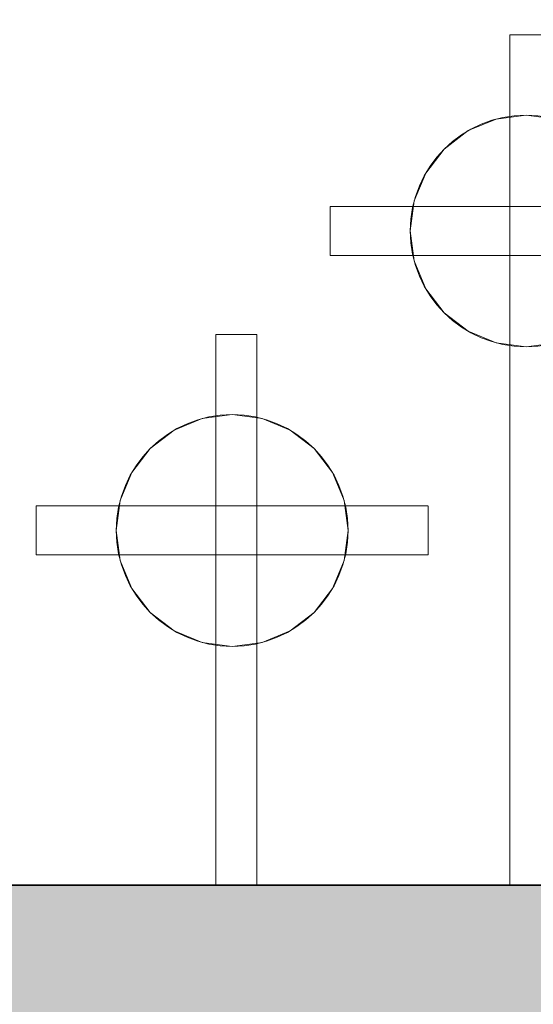
# Model space of a CAD drawing. Units: inches. Extents: x 2696 to 3240, y 1564 to 2310.
# Tile 30 of 76: x 3142.316 to 3146.244, y 1698.791 to 1706.319. Entities that reach past the tile are written whole.
import ezdxf

# ---------------------------------------------------------------- set-up
doc = ezdxf.new("R2010")
doc.units = ezdxf.units.IN
for name, color, linetype, lineweight in [('A-ANNO-DIMS', 3, 'Continuous', 18), ('A-FLOR-FIXT', 8, 'Continuous', 18), ('A-FURN', 251, 'Continuous', 13), ('A-WALL', 7, 'Continuous', 35), ('A-WALL-PATT', 9, 'Continuous', 13)]:
    doc.layers.add(name, color=color, linetype=linetype, lineweight=lineweight)
doc.layers.add('FURNITURE', color=250, linetype='Continuous')
doc.styles.add('TIMES NEW', font='times.ttf')
doc.dimstyles.new('Siddhuu', dxfattribs={"dimtxt": 6, "dimasz": 2.5, "dimexe": 1.25, "dimexo": 0.625, "dimtad": 1, "dimdec": 1, "dimlunit": 4, "dimtxsty": 'TIMES NEW', "dimcen": 2.5, "dimclrd": 256, "dimclre": 1, "dimclrt": 7, "dimadec": 0, "dimazin": 0, "dimtfac": 1, "dimtdec": 1, "dimtmove": 0, "dimatfit": 3, "dimfxl": 1, "dimtolj": 1, "dimlwd": -1, "dimarcsym": 0})

# ---------------------------------------------------------------- blocks, each defined once
blk = doc.blocks.new('A$C1af1f523')
at = {"layer": 'A-FURN'}
for p, q in [((-2.9003, 3.9351), (-2.9003, 0.9365)), ((-2.9003, 3.9351, 0.5), (-2.9003, 0.9365, 0.5)), ((-2.9003, 3.9351), (-2.9003, 3.9351, 0.5)), ((-2.5253, 3.9351), (-2.9003, 3.9351)), ((-2.5253, 3.9351, 0.5), (-2.9003, 3.9351, 0.5)), ((-2.5253, 3.9351), (-2.5253, 0.9365)), ((-2.5253, 3.9351, 0.5), (-2.5253, 0.9365, 0.5)), ((-2.5253, 3.9351), (-2.5253, 3.9351, 0.5)), ((-2.7128, 3.3215), (-2.7128, 3.3215, 0.5)), ((-2.9421, 3.2913), (-2.9421, 3.2913, 0.5)), ((-2.4835, 3.2913), (-2.4835, 3.2913, 0.5)), ((-3.1558, 3.2028), (-3.1558, 3.2028, 0.5)), ((-2.2698, 3.2028), (-2.2698, 3.2028, 0.5)), ((-3.3393, 3.062), (-3.3393, 3.062, 0.5)), ((-2.0863, 3.062), (-2.0863, 3.062, 0.5)), ((-3.4801, 2.8785), (-3.4801, 2.8785, 0.5)), ((-1.9455, 2.8785), (-1.9455, 2.8785, 0.5)), ((-3.5686, 2.6648), (-3.5686, 2.6648, 0.5)), ((-1.857, 2.6648), (-1.857, 2.6648, 0.5)), ((0, 2.5605), (-4.2116, 2.5605)), ((0, 2.5605, 0.5), (-4.2116, 2.5605, 0.5)), ((-4.2116, 2.5605), (-4.2116, 2.5605, 0.5)), ((-4.2116, 2.5594), (-4.2116, 2.248)), ((-4.2116, 2.5594, 0.5), (-4.2116, 2.248, 0.5)), ((-4.2116, 2.5594), (-4.2116, 2.5594, 0.5)), ((-3.5988, 2.4355), (-3.5988, 2.4355, 0.5)), ((-1.8268, 2.4355), (-1.8268, 2.4355, 0.5)), ((0, 2.248), (-4.2116, 2.248)), ((0, 2.248, 0.5), (-4.2116, 2.248, 0.5)), ((-4.2116, 2.248), (-4.2116, 2.248, 0.5)), ((-4.2116, 2.248), (-4.2116, 2.2469)), ((-4.2116, 2.248, 0.5), (-4.2116, 2.2469, 0.5)), ((-4.2116, 2.2469), (-4.2116, 2.2469, 0.5)), ((-3.5686, 2.2061), (-3.5686, 2.2061, 0.5)), ((-1.857, 2.2061), (-1.857, 2.2061, 0.5)), ((-3.4801, 1.9924), (-3.4801, 1.9924, 0.5)), ((-1.9455, 1.9924), (-1.9455, 1.9924, 0.5)), ((-3.3393, 1.8089), (-3.3393, 1.8089, 0.5)), ((-2.0863, 1.8089), (-2.0863, 1.8089, 0.5)), ((-4.8156, 1.6871), (-5.1906, 1.6871)), ((-4.8156, 1.6871, 0.5), (-5.1906, 1.6871, 0.5)), ((-5.1906, 1.6871), (-5.1906, 1.6871, 0.5)), ((-5.1906, 1.6871), (-5.1901, -1.3115)), ((-5.1906, 1.6871, 0.5), (-5.1901, -1.3115, 0.5)), ((-4.8156, 1.6871), (-4.8156, 1.6871, 0.5)), ((-4.8156, 1.6871), (-4.8151, -1.3115)), ((-4.8156, 1.6871, 0.5), (-4.8151, -1.3115, 0.5)), ((-3.1558, 1.6681), (-3.1558, 1.6681, 0.5)), ((-2.2698, 1.6681), (-2.2698, 1.6681, 0.5)), ((-2.9421, 1.5796), (-2.9421, 1.5796, 0.5)), ((-2.7128, 1.5494), (-2.7128, 1.5494, 0.5)), ((-2.4835, 1.5796), (-2.4835, 1.5796, 0.5)), ((-5.0026, 1.0735), (-5.0026, 1.0735, 0.5)), ((-5.232, 1.0433), (-5.232, 1.0433, 0.5)), ((-4.7733, 1.0433), (-4.7733, 1.0433, 0.5)), ((-5.4457, 0.9548), (-5.4457, 0.9548, 0.5)), ((-4.5596, 0.9548), (-4.5596, 0.9548, 0.5)), ((-2.9003, 0.9365), (-2.9003, 0.9365, 0.5)), ((-2.5253, 0.9365), (-2.8979, 0.9365)), ((-2.5253, 0.9365, 0.5), (-2.8979, 0.9365, 0.5)), ((-2.8979, 0.9365), (-2.8979, 0.9365, 0.5)), ((-2.5253, 0.9365), (-2.5253, 0.9365, 0.5)), ((-5.6292, 0.814), (-5.6292, 0.814, 0.5)), ((-4.3761, 0.814), (-4.3761, 0.814, 0.5)), ((-5.77, 0.6305), (-5.77, 0.6305, 0.5)), ((-4.2353, 0.6305), (-4.2353, 0.6305, 0.5)), ((-5.8585, 0.4168), (-5.8585, 0.4168, 0.5)), ((-4.1468, 0.4168), (-4.1468, 0.4168, 0.5)), ((0, 0.3125), (-6.5015, 0.3125)), ((0, 0.3125, 0.5), (-6.5015, 0.3125, 0.5)), ((-6.5015, 0.3125), (-6.5015, 0.3125, 0.5)), ((-6.5015, 0.3114), (-6.5015, 0)), ((-6.5015, 0.3114, 0.5), (-6.5015, 0, 0.5)), ((-6.5015, 0.3114), (-6.5015, 0.3114, 0.5)), ((-5.8887, 0.1875), (-5.8887, 0.1875, 0.5)), ((-4.1166, 0.1875), (-4.1166, 0.1875, 0.5))]:
    blk.add_line(p, q, dxfattribs=at)
for centre in [(-2.7128, 2.4355), (-2.7128, 2.4355, 0.5), (-5.0026, 0.1875), (-5.0026, 0.1875, 0.5)]:
    blk.add_circle(centre, 0.886, dxfattribs=at)
at = {"layer": 'FURNITURE'}
for p, q in [((0, 2.5605), (0, 2.5605, 0.5)), ((0, 2.248), (0, 2.248, 0.5)), ((0, 0.3125), (0, 0.3125, 0.5))]:
    blk.add_line(p, q, dxfattribs=at)
at = {"layer": 'A-FURN'}
mesh = blk.add_polyface(dxfattribs=at)
corners = [(-2.9003, 0.9365, 0.5), (-2.9003, 3.9351), (-2.9003, 0.9365), (-2.9003, 3.9351, 0.5)]
mesh.append_faces([[corners[k] for k in face] for face in [(2, 1, 0), (3, 0, 1)]], dxfattribs={"vtx1": -1})
mesh = blk.add_polyface(dxfattribs=at)
corners = [(-2.5253, 3.9351, 0.5), (-2.9003, 3.9351), (-2.9003, 3.9351, 0.5), (-2.5253, 3.9351)]
mesh.append_faces([[corners[k] for k in face] for face in [(2, 1, 0), (3, 0, 1)]], dxfattribs={"vtx1": -1})
mesh = blk.add_polyface(dxfattribs=at)
corners = [(-2.5253, 0.9365, 0.5), (-2.5253, 3.9351), (-2.5253, 0.9365), (-2.5253, 3.9351, 0.5)]
mesh.append_faces([[corners[k] for k in face] for face in [(2, 1, 0), (3, 0, 1)]], dxfattribs={"vtx1": -1})
mesh = blk.add_polyface(dxfattribs=at)
corners = [(-2.7128, 3.3215), (-2.9421, 3.2913, 0.5), (-2.9421, 3.2913), (-2.7128, 3.3215, 0.5)]
mesh.append_faces([[corners[k] for k in face] for face in [(2, 1, 0), (3, 0, 1)]], dxfattribs={"vtx1": -1})
mesh = blk.add_polyface(dxfattribs=at)
corners = [(-2.4835, 3.2913), (-2.7128, 3.3215, 0.5), (-2.7128, 3.3215), (-2.4835, 3.2913, 0.5)]
mesh.append_faces([[corners[k] for k in face] for face in [(2, 1, 0), (3, 0, 1)]], dxfattribs={"vtx1": -1})
mesh = blk.add_polyface(dxfattribs=at)
corners = [(-2.9421, 3.2913), (-3.1558, 3.2028, 0.5), (-3.1558, 3.2028), (-2.9421, 3.2913, 0.5)]
mesh.append_faces([[corners[k] for k in face] for face in [(2, 1, 0), (3, 0, 1)]], dxfattribs={"vtx1": -1})
mesh = blk.add_polyface(dxfattribs=at)
corners = [(-2.2698, 3.2028), (-2.4835, 3.2913, 0.5), (-2.4835, 3.2913), (-2.2698, 3.2028, 0.5)]
mesh.append_faces([[corners[k] for k in face] for face in [(2, 1, 0), (3, 0, 1)]], dxfattribs={"vtx1": -1})
mesh = blk.add_polyface(dxfattribs=at)
corners = [(-3.1558, 3.2028), (-3.3393, 3.062, 0.5), (-3.3393, 3.062), (-3.1558, 3.2028, 0.5)]
mesh.append_faces([[corners[k] for k in face] for face in [(2, 1, 0), (3, 0, 1)]], dxfattribs={"vtx1": -1})
mesh = blk.add_polyface(dxfattribs=at)
corners = [(-2.0863, 3.062), (-2.2698, 3.2028, 0.5), (-2.2698, 3.2028), (-2.0863, 3.062, 0.5)]
mesh.append_faces([[corners[k] for k in face] for face in [(2, 1, 0), (3, 0, 1)]], dxfattribs={"vtx1": -1})
mesh = blk.add_polyface(dxfattribs=at)
corners = [(-3.3393, 3.062, 0.5), (-3.4801, 2.8785), (-3.3393, 3.062), (-3.4801, 2.8785, 0.5)]
mesh.append_faces([[corners[k] for k in face] for face in [(2, 1, 0), (3, 0, 1)]], dxfattribs={"vtx1": -1})
mesh = blk.add_polyface(dxfattribs=at)
corners = [(-1.9455, 2.8785, 0.5), (-2.0863, 3.062), (-1.9455, 2.8785), (-2.0863, 3.062, 0.5)]
mesh.append_faces([[corners[k] for k in face] for face in [(2, 1, 0), (3, 0, 1)]], dxfattribs={"vtx1": -1})
mesh = blk.add_polyface(dxfattribs=at)
corners = [(-3.4801, 2.8785, 0.5), (-3.5686, 2.6648), (-3.4801, 2.8785), (-3.5686, 2.6648, 0.5)]
mesh.append_faces([[corners[k] for k in face] for face in [(2, 1, 0), (3, 0, 1)]], dxfattribs={"vtx1": -1})
mesh = blk.add_polyface(dxfattribs=at)
corners = [(-1.857, 2.6648, 0.5), (-1.9455, 2.8785), (-1.857, 2.6648), (-1.9455, 2.8785, 0.5)]
mesh.append_faces([[corners[k] for k in face] for face in [(2, 1, 0), (3, 0, 1)]], dxfattribs={"vtx1": -1})
mesh = blk.add_polyface(dxfattribs=at)
corners = [(-3.5686, 2.6648, 0.5), (-3.5988, 2.4355), (-3.5686, 2.6648), (-3.5988, 2.4355, 0.5)]
mesh.append_faces([[corners[k] for k in face] for face in [(2, 1, 0), (3, 0, 1)]], dxfattribs={"vtx1": -1})
mesh = blk.add_polyface(dxfattribs=at)
corners = [(-1.8268, 2.4355, 0.5), (-1.857, 2.6648), (-1.8268, 2.4355), (-1.857, 2.6648, 0.5)]
mesh.append_faces([[corners[k] for k in face] for face in [(2, 1, 0), (3, 0, 1)]], dxfattribs={"vtx1": -1})
mesh = blk.add_polyface(dxfattribs=at)
corners = [(0, 2.5605, 0.5), (-4.2116, 2.5605), (-4.2116, 2.5605, 0.5), (0, 2.5605)]
mesh.append_faces([[corners[k] for k in face] for face in [(2, 1, 0), (3, 0, 1)]], dxfattribs={"vtx1": -1})
mesh = blk.add_polyface(dxfattribs=at)
corners = [(-4.2116, 2.2469, 0.5), (-4.2116, 2.248), (-4.2116, 2.2469), (-4.2116, 2.5594), (-4.2116, 2.5594, 0.5), (-4.2116, 2.248, 0.5)]
mesh.append_faces([[corners[k] for k in face] for face in [(3, 0, 1), (4, 0, 3)]], dxfattribs={"vtx0": -1, "vtx1": -1})
mesh.append_faces([[corners[k] for k in face] for face in [(2, 1, 0), (5, 0, 4)]], dxfattribs={"vtx1": -1})
mesh = blk.add_polyface(dxfattribs=at)
corners = [(-3.5988, 2.4355, 0.5), (-3.5686, 2.2061), (-3.5988, 2.4355), (-3.5686, 2.2061, 0.5)]
mesh.append_faces([[corners[k] for k in face] for face in [(2, 1, 0), (3, 0, 1)]], dxfattribs={"vtx1": -1})
mesh = blk.add_polyface(dxfattribs=at)
corners = [(-1.857, 2.2061, 0.5), (-1.8268, 2.4355), (-1.857, 2.2061), (-1.8268, 2.4355, 0.5)]
mesh.append_faces([[corners[k] for k in face] for face in [(2, 1, 0), (3, 0, 1)]], dxfattribs={"vtx1": -1})
mesh = blk.add_polyface(dxfattribs=at)
corners = [(0, 2.248, 0.5), (-4.2116, 2.248), (-4.2116, 2.248, 0.5), (0, 2.248)]
mesh.append_faces([[corners[k] for k in face] for face in [(2, 1, 0), (3, 0, 1)]], dxfattribs={"vtx1": -1})
mesh = blk.add_polyface(dxfattribs=at)
corners = [(-3.5686, 2.2061, 0.5), (-3.4801, 1.9924), (-3.5686, 2.2061), (-3.4801, 1.9924, 0.5)]
mesh.append_faces([[corners[k] for k in face] for face in [(2, 1, 0), (3, 0, 1)]], dxfattribs={"vtx1": -1})
mesh = blk.add_polyface(dxfattribs=at)
corners = [(-1.9455, 1.9924, 0.5), (-1.857, 2.2061), (-1.9455, 1.9924), (-1.857, 2.2061, 0.5)]
mesh.append_faces([[corners[k] for k in face] for face in [(2, 1, 0), (3, 0, 1)]], dxfattribs={"vtx1": -1})
mesh = blk.add_polyface(dxfattribs=at)
corners = [(-3.4801, 1.9924, 0.5), (-3.3393, 1.8089), (-3.4801, 1.9924), (-3.3393, 1.8089, 0.5)]
mesh.append_faces([[corners[k] for k in face] for face in [(2, 1, 0), (3, 0, 1)]], dxfattribs={"vtx1": -1})
mesh = blk.add_polyface(dxfattribs=at)
corners = [(-2.0863, 1.8089, 0.5), (-1.9455, 1.9924), (-2.0863, 1.8089), (-1.9455, 1.9924, 0.5)]
mesh.append_faces([[corners[k] for k in face] for face in [(2, 1, 0), (3, 0, 1)]], dxfattribs={"vtx1": -1})
mesh = blk.add_polyface(dxfattribs=at)
corners = [(-3.1558, 1.6681, 0.5), (-3.3393, 1.8089), (-3.3393, 1.8089, 0.5), (-3.1558, 1.6681)]
mesh.append_faces([[corners[k] for k in face] for face in [(2, 1, 0), (3, 0, 1)]], dxfattribs={"vtx1": -1})
mesh = blk.add_polyface(dxfattribs=at)
corners = [(-2.0863, 1.8089, 0.5), (-2.2698, 1.6681), (-2.2698, 1.6681, 0.5), (-2.0863, 1.8089)]
mesh.append_faces([[corners[k] for k in face] for face in [(2, 1, 0), (3, 0, 1)]], dxfattribs={"vtx1": -1})
mesh = blk.add_polyface(dxfattribs=at)
corners = [(-4.8156, 1.6871, 0.5), (-5.1906, 1.6871), (-5.1906, 1.6871, 0.5), (-4.8156, 1.6871)]
mesh.append_faces([[corners[k] for k in face] for face in [(2, 1, 0), (3, 0, 1)]], dxfattribs={"vtx1": -1})
mesh = blk.add_polyface(dxfattribs=at)
corners = [(-5.1901, -1.3115, 0.5), (-5.1906, 1.6871), (-5.1901, -1.3115), (-5.1906, 1.6871, 0.5)]
mesh.append_faces([[corners[k] for k in face] for face in [(2, 1, 0), (3, 0, 1)]], dxfattribs={"vtx1": -1})
mesh = blk.add_polyface(dxfattribs=at)
corners = [(-4.8151, -1.3115, 0.5), (-4.8156, 1.6871), (-4.8151, -1.3115), (-4.8156, 1.6871, 0.5)]
mesh.append_faces([[corners[k] for k in face] for face in [(2, 1, 0), (3, 0, 1)]], dxfattribs={"vtx1": -1})
mesh = blk.add_polyface(dxfattribs=at)
corners = [(-2.9421, 1.5796, 0.5), (-3.1558, 1.6681), (-3.1558, 1.6681, 0.5), (-2.9421, 1.5796)]
mesh.append_faces([[corners[k] for k in face] for face in [(2, 1, 0), (3, 0, 1)]], dxfattribs={"vtx1": -1})
mesh = blk.add_polyface(dxfattribs=at)
corners = [(-2.2698, 1.6681, 0.5), (-2.4835, 1.5796), (-2.4835, 1.5796, 0.5), (-2.2698, 1.6681)]
mesh.append_faces([[corners[k] for k in face] for face in [(2, 1, 0), (3, 0, 1)]], dxfattribs={"vtx1": -1})
mesh = blk.add_polyface(dxfattribs=at)
corners = [(-2.7128, 1.5494, 0.5), (-2.9421, 1.5796), (-2.9421, 1.5796, 0.5), (-2.7128, 1.5494)]
mesh.append_faces([[corners[k] for k in face] for face in [(2, 1, 0), (3, 0, 1)]], dxfattribs={"vtx1": -1})
mesh = blk.add_polyface(dxfattribs=at)
corners = [(-2.4835, 1.5796, 0.5), (-2.7128, 1.5494), (-2.7128, 1.5494, 0.5), (-2.4835, 1.5796)]
mesh.append_faces([[corners[k] for k in face] for face in [(2, 1, 0), (3, 0, 1)]], dxfattribs={"vtx1": -1})
mesh = blk.add_polyface(dxfattribs=at)
corners = [(-5.0026, 1.0735), (-5.232, 1.0433, 0.5), (-5.232, 1.0433), (-5.0026, 1.0735, 0.5)]
mesh.append_faces([[corners[k] for k in face] for face in [(2, 1, 0), (3, 0, 1)]], dxfattribs={"vtx1": -1})
mesh = blk.add_polyface(dxfattribs=at)
corners = [(-4.7733, 1.0433), (-5.0026, 1.0735, 0.5), (-5.0026, 1.0735), (-4.7733, 1.0433, 0.5)]
mesh.append_faces([[corners[k] for k in face] for face in [(2, 1, 0), (3, 0, 1)]], dxfattribs={"vtx1": -1})
mesh = blk.add_polyface(dxfattribs=at)
corners = [(-5.232, 1.0433), (-5.4457, 0.9548, 0.5), (-5.4457, 0.9548), (-5.232, 1.0433, 0.5)]
mesh.append_faces([[corners[k] for k in face] for face in [(2, 1, 0), (3, 0, 1)]], dxfattribs={"vtx1": -1})
mesh = blk.add_polyface(dxfattribs=at)
corners = [(-4.5596, 0.9548), (-4.7733, 1.0433, 0.5), (-4.7733, 1.0433), (-4.5596, 0.9548, 0.5)]
mesh.append_faces([[corners[k] for k in face] for face in [(2, 1, 0), (3, 0, 1)]], dxfattribs={"vtx1": -1})
mesh = blk.add_polyface(dxfattribs=at)
corners = [(-5.4457, 0.9548), (-5.6292, 0.814, 0.5), (-5.6292, 0.814), (-5.4457, 0.9548, 0.5)]
mesh.append_faces([[corners[k] for k in face] for face in [(2, 1, 0), (3, 0, 1)]], dxfattribs={"vtx1": -1})
mesh = blk.add_polyface(dxfattribs=at)
corners = [(-4.3761, 0.814), (-4.5596, 0.9548, 0.5), (-4.5596, 0.9548), (-4.3761, 0.814, 0.5)]
mesh.append_faces([[corners[k] for k in face] for face in [(2, 1, 0), (3, 0, 1)]], dxfattribs={"vtx1": -1})
mesh = blk.add_polyface(dxfattribs=at)
corners = [(-2.5253, 0.9365, 0.5), (-2.8979, 0.9365), (-2.8979, 0.9365, 0.5), (-2.5253, 0.9365)]
mesh.append_faces([[corners[k] for k in face] for face in [(2, 1, 0), (3, 0, 1)]], dxfattribs={"vtx1": -1})
mesh = blk.add_polyface(dxfattribs=at)
corners = [(-5.6292, 0.814, 0.5), (-5.77, 0.6305), (-5.6292, 0.814), (-5.77, 0.6305, 0.5)]
mesh.append_faces([[corners[k] for k in face] for face in [(2, 1, 0), (3, 0, 1)]], dxfattribs={"vtx1": -1})
mesh = blk.add_polyface(dxfattribs=at)
corners = [(-4.2353, 0.6305, 0.5), (-4.3761, 0.814), (-4.2353, 0.6305), (-4.3761, 0.814, 0.5)]
mesh.append_faces([[corners[k] for k in face] for face in [(2, 1, 0), (3, 0, 1)]], dxfattribs={"vtx1": -1})
mesh = blk.add_polyface(dxfattribs=at)
corners = [(-5.77, 0.6305, 0.5), (-5.8585, 0.4168), (-5.77, 0.6305), (-5.8585, 0.4168, 0.5)]
mesh.append_faces([[corners[k] for k in face] for face in [(2, 1, 0), (3, 0, 1)]], dxfattribs={"vtx1": -1})
mesh = blk.add_polyface(dxfattribs=at)
corners = [(-4.1468, 0.4168, 0.5), (-4.2353, 0.6305), (-4.1468, 0.4168), (-4.2353, 0.6305, 0.5)]
mesh.append_faces([[corners[k] for k in face] for face in [(2, 1, 0), (3, 0, 1)]], dxfattribs={"vtx1": -1})
mesh = blk.add_polyface(dxfattribs=at)
corners = [(-5.8585, 0.4168, 0.5), (-5.8887, 0.1875), (-5.8585, 0.4168), (-5.8887, 0.1875, 0.5)]
mesh.append_faces([[corners[k] for k in face] for face in [(2, 1, 0), (3, 0, 1)]], dxfattribs={"vtx1": -1})
mesh = blk.add_polyface(dxfattribs=at)
corners = [(-4.1166, 0.1875, 0.5), (-4.1468, 0.4168), (-4.1166, 0.1875), (-4.1468, 0.4168, 0.5)]
mesh.append_faces([[corners[k] for k in face] for face in [(2, 1, 0), (3, 0, 1)]], dxfattribs={"vtx1": -1})
mesh = blk.add_polyface(dxfattribs=at)
corners = [(0, 0.3125, 0.5), (-6.5015, 0.3125), (-6.5015, 0.3125, 0.5), (0, 0.3125)]
mesh.append_faces([[corners[k] for k in face] for face in [(2, 1, 0), (3, 0, 1)]], dxfattribs={"vtx1": -1})
mesh = blk.add_polyface(dxfattribs=at)
corners = [(-6.5015, -0.0011, 0.5), (-6.5015, 0), (-6.5015, -0.0011), (-6.5015, 0.3114), (-6.5015, 0.3114, 0.5), (-6.5015, 0, 0.5)]
mesh.append_faces([[corners[k] for k in face] for face in [(3, 0, 1), (4, 0, 3)]], dxfattribs={"vtx0": -1, "vtx1": -1})
mesh.append_faces([[corners[k] for k in face] for face in [(2, 1, 0), (5, 0, 4)]], dxfattribs={"vtx1": -1})
mesh = blk.add_polyface(dxfattribs=at)
corners = [(-5.8887, 0.1875, 0.5), (-5.8585, -0.0418), (-5.8887, 0.1875), (-5.8585, -0.0418, 0.5)]
mesh.append_faces([[corners[k] for k in face] for face in [(2, 1, 0), (3, 0, 1)]], dxfattribs={"vtx1": -1})
mesh = blk.add_polyface(dxfattribs=at)
corners = [(-4.1468, -0.0418, 0.5), (-4.1166, 0.1875), (-4.1468, -0.0418), (-4.1166, 0.1875, 0.5)]
mesh.append_faces([[corners[k] for k in face] for face in [(2, 1, 0), (3, 0, 1)]], dxfattribs={"vtx1": -1})
blk = doc.blocks.new('*D51')
at = {"layer": 'A-ANNO-DIMS', "color": 1, "lineweight": -2, "transparency": 16777216}
for p, q in [((3016.6114, 1979.5761), (3016.6114, 1568.9511)), ((3148.6114, 1979.5761), (3148.6114, 1568.9511))]:
    blk.add_line(p, q, dxfattribs=at)
at = {"layer": 'A-ANNO-DIMS', "transparency": 16777216}
blk.add_line((3019.1114, 1570.2011), (3146.1114, 1570.2011), dxfattribs=at)
for points in [[(3019.1114, 1570.6178), (3019.1114, 1569.7844), (3016.6114, 1570.2011)], [(3146.1114, 1570.6178), (3146.1114, 1569.7844), (3148.6114, 1570.2011)]]:
    blk.add_solid(points, dxfattribs=at)
at = {"layer": 'Defpoints', "color": 0, "transparency": 16777216}
for p in [(3016.6114, 1980.2011), (3148.6114, 1980.2011), (3148.6114, 1570.2011)]:
    blk.add_point(p, dxfattribs=at)
at = {"layer": 'A-ANNO-DIMS', "color": 7, "transparency": 16777216, "insert": (3082.6114, 1573.878), "char_height": 6, "attachment_point": 5, "style": 'TIMES NEW'}
blk.add_mtext('\\A1;11\'-0"', dxfattribs=at)
blk = doc.blocks.new('*D56')
at = {"layer": 'A-ANNO-DIMS', "color": 1, "lineweight": -2, "transparency": 16777216}
for p, q in [((2966.3338, 1884.2011), (3235.8614, 1884.2011)), ((2966.3338, 1665.2011), (3235.8614, 1665.2011))]:
    blk.add_line(p, q, dxfattribs=at)
at = {"layer": 'A-ANNO-DIMS', "transparency": 16777216}
blk.add_line((3234.6114, 1667.7011), (3234.6114, 1881.7011), dxfattribs=at)
for points in [[(3234.1947, 1881.7011), (3235.0281, 1881.7011), (3234.6114, 1884.2011)], [(3234.1947, 1667.7011), (3235.0281, 1667.7011), (3234.6114, 1665.2011)]]:
    blk.add_solid(points, dxfattribs=at)
at = {"layer": 'Defpoints', "color": 0, "transparency": 16777216}
for p in [(2965.7088, 1884.2011), (3234.6114, 1884.2011), (2965.7088, 1665.2011)]:
    blk.add_point(p, dxfattribs=at)
at = {"layer": 'A-ANNO-DIMS', "color": 7, "transparency": 16777216, "insert": (3230.9345, 1774.7011), "char_height": 6, "attachment_point": 5, "rotation": 90, "style": 'TIMES NEW'}
blk.add_mtext('\\A1;18\'-3"', dxfattribs=at)

msp = doc.modelspace()

# ---------------------------------------------------------------- hatches: boundary and pattern name
at = {"layer": 'A-WALL-PATT', "transparency": 33554556}
h = msp.add_hatch(color=256, dxfattribs=at)
h.dxf.hatch_style = 1
h.paths.add_polyline_path([(2879.1114, 2253.2011), (2905.9101, 2253.2011), (2905.9101, 2262.2011), (2841.889, 2262.2011), (2841.889, 2253.2011), (2870.1114, 2253.2011), (2870.1114, 2176.6011), (2965.7088, 2176.6011), (2965.7088, 2206.7011), (2973.5828, 2206.7011), (2973.5828, 2215.7011), (2965.7088, 2215.7011), (2965.7088, 2262.2011), (2929.9101, 2262.2011), (2929.9101, 2253.2011), (2956.7088, 2253.2011), (2956.7088, 2185.6011), (2879.1114, 2185.6011)])
h.paths.add_polyline_path([(2782.8338, 2262.2011), (2745.6114, 2262.2011), (2745.6114, 2228.7287), (2754.6114, 2228.7287), (2754.6114, 2253.2011), (2782.8338, 2253.2011)])
h.paths.add_polyline_path([(2754.6114, 2136.2011), (2965.7088, 2136.2011), (2965.7088, 2145.2011), (2879.1114, 2145.2011), (2879.1114, 2147.0735), (2877.3397, 2147.0735), (2870.1114, 2147.0735), (2870.1114, 2145.2011), (2754.6114, 2145.2011), (2754.6114, 2169.6735), (2745.6114, 2169.6735), (2745.6114, 2000.2011), (2754.6114, 2000.2011), (2754.6114, 2019.2011), (2849.0828, 2019.2011), (2849.0828, 2023.7011), (2841.2088, 2023.7011), (2841.2088, 2051.8271), (2836.7088, 2051.8271), (2836.7088, 2023.7011), (2754.6114, 2023.7011), (2754.6114, 2091.2011), (2836.7088, 2091.2011), (2836.7088, 2087.8271), (2841.2088, 2087.8271), (2841.2088, 2095.7011), (2754.6114, 2095.7011)])
h.paths.add_polyline_path([(2965.7088, 2136.2011), (2956.7088, 2136.2011), (2956.7088, 2023.7011), (2885.0828, 2023.7011), (2885.0828, 2019.2011), (2956.7088, 2019.2011), (2956.7088, 1950.5751), (2965.7088, 1950.5751), (2965.7088, 1980.2011), (2973.5828, 1980.2011), (2973.5828, 1989.2011), (2965.7088, 1989.2011)])
h.paths.add_polyline_path([(2754.6114, 1906.7011), (2880.2088, 1906.7011), (2884.7088, 1906.7011), (2956.7088, 1906.7011), (2956.7088, 1792.7011), (2944.7088, 1792.7011), (2944.7088, 1783.7011), (2956.7088, 1783.7011), (2956.7088, 1740.2011), (2884.7088, 1740.2011), (2884.7088, 1783.7011), (2896.7088, 1783.7011), (2896.7088, 1792.7011), (2884.7088, 1792.7011), (2884.7088, 1846.7011), (2880.2088, 1846.7011), (2880.2088, 1740.2011), (2754.6114, 1740.2011), (2754.6114, 1777.2011), (2745.6114, 1777.2011), (2745.6114, 1692.7011), (2754.6114, 1692.7011), (2754.6114, 1731.2011), (2956.7088, 1731.2011), (2956.7088, 1723.3271), (2965.7088, 1723.3271), (2965.7088, 1884.2011), (2973.5828, 1884.2011), (2973.5828, 1893.2011), (2965.7088, 1893.2011), (2965.7088, 1914.5751), (2956.7088, 1914.5751), (2956.7088, 1911.2011), (2754.6114, 1911.2011), (2754.6114, 1930.2011), (2745.6114, 1930.2011), (2745.6114, 1817.2011), (2754.6114, 1817.2011), (2754.6114, 1854.2011), (2826.6114, 1854.2011), (2826.6114, 1868.8271), (2822.1114, 1868.8271), (2822.1114, 1858.7011), (2754.6114, 1858.7011)])
h.paths.add_polyline_path([(2965.7088, 1656.2011), (3008.2374, 1656.2011), (3008.2374, 1665.2011), (2965.7088, 1665.2011), (2965.7088, 1693.3271), (2956.7088, 1693.3271), (2956.7088, 1686.2011), (2934.5828, 1686.2011), (2934.5828, 1681.7011), (2956.7088, 1681.7011), (2956.7088, 1614.2011), (2896.7088, 1614.2011), (2896.7088, 1681.7011), (2904.5828, 1681.7011), (2904.5828, 1686.2011), (2892.2088, 1686.2011), (2892.2088, 1614.2011), (2858.4101, 1614.2011), (2858.4101, 1605.2011), (2965.7088, 1605.2011)])
h.paths.add_polyline_path([(2788.4101, 1614.2011), (2754.6114, 1614.2011), (2754.6114, 1652.7011), (2745.6114, 1652.7011), (2745.6114, 1605.2011), (2788.4101, 1605.2011)])
h.paths.add_polyline_path([(3199.6114, 1633.0476), (3190.6114, 1633.0476), (3190.6114, 1614.2011), (3082.6114, 1614.2011), (3082.6114, 1665.2011), (3070.2374, 1665.2011), (3070.2374, 1656.2011), (3078.1114, 1656.2011), (3078.1114, 1605.2011), (3199.6114, 1605.2011)])
h.paths.add_polyline_path([(3199.6114, 1702.0476), (3190.6114, 1702.0476), (3190.6114, 1699.7011), (3106.6114, 1699.7011), (3106.6114, 1747.7011), (3190.6114, 1747.7011), (3190.6114, 1752.2011), (3082.6114, 1752.2011), (3082.6114, 1760.0751), (3078.1114, 1760.0751), (3078.1114, 1747.7011), (3102.1114, 1747.7011), (3102.1114, 1699.7011), (3078.1114, 1699.7011), (3078.1114, 1695.2011), (3190.6114, 1695.2011), (3190.6114, 1676.3546), (3199.6114, 1676.3546)])
h.paths.add_polyline_path([(3199.6114, 1783.2011), (3190.6114, 1783.2011), (3190.6114, 1745.3546), (3199.6114, 1745.3546)])
h.paths.add_polyline_path([(3082.6114, 1884.2011), (3190.6114, 1884.2011), (3190.6114, 1853.2011), (3199.6114, 1853.2011), (3199.6114, 1901.7011), (3190.6114, 1901.7011), (3190.6114, 1893.2011), (3005.5828, 1893.2011), (3005.5828, 1891.2811), (3005.5828, 1884.2011), (3078.1114, 1884.2011), (3078.1114, 1792.0751), (3082.6114, 1792.0751)])
h.paths.add_polyline_path([(3199.6114, 1994.7011), (3190.6114, 1994.7011), (3190.6114, 1989.2011), (3073.7088, 1989.2011), (3073.7088, 2034.2011), (3069.2088, 2034.2011), (3069.2088, 1989.2011), (3005.5828, 1989.2011), (3005.5828, 1980.2011), (3190.6114, 1980.2011), (3190.6114, 1971.7011), (3199.6114, 1971.7011)])
h.paths.add_polyline_path([(3199.6114, 2155.2011), (3190.6114, 2155.2011), (3190.6114, 2064.7011), (3199.6114, 2064.7011)])
h.paths.add_polyline_path([(3190.6114, 2074.7011), (3106.6114, 2074.7011), (3106.6114, 2122.7011), (3190.6114, 2122.7011), (3190.6114, 2127.2011), (3082.7088, 2127.2011), (3082.7088, 2135.0751), (3073.7088, 2135.0751), (3073.7088, 2122.7011), (3102.1114, 2122.7011), (3102.1114, 2074.7011), (3069.2088, 2074.7011), (3069.2088, 2070.2011), (3190.6114, 2070.2011)])
h.paths.add_polyline_path([(3082.7088, 2253.2011), (3190.6114, 2253.2011), (3190.6114, 2225.2011), (3199.6114, 2225.2011), (3199.6114, 2262.2011), (3073.7088, 2262.2011), (3073.7088, 2215.7011), (3035.5828, 2215.7011), (3035.5828, 2206.7011), (3073.7088, 2206.7011), (3073.7088, 2171.0751), (3082.7088, 2171.0751)])

# ---------------------------------------------------------------- linework, layer by layer
at = {"layer": 'A-WALL'}
msp.add_line((3106.6114, 1699.7011), (3190.6114, 1699.7011), dxfattribs=at)

# ---------------------------------------------------------------- block references
at = {"layer": 'A-FLOR-FIXT', "xscale": -1, "rotation": 90}
msp.add_blockref('A$C1af1f523', (3146.3764, 1699.7011), dxfattribs=at)

# ---------------------------------------------------------------- dimensions: what is measured, and where the dimension line sits
at = {"layer": 'A-ANNO-DIMS'}
dim = msp.add_linear_dim(base=(3148.6114, 1570.2011), p1=(3016.6114, 1980.2011), p2=(3148.6114, 1980.2011), dimstyle='Siddhuu', override={"dimdec": 1, "dimlfac": 1, "dimrnd": 0, "dimzin": 1, "dimdsep": 46, "dimlunit": 4, "dimfrac": 2}, dxfattribs=at)
dim.commit()
dim.dimension.update_dxf_attribs({"geometry": '*D51', "text_midpoint": (3082.6114, 1573.878)})
dim = msp.add_linear_dim(base=(3234.6114, 1884.2011), p1=(2965.7088, 1665.2011), p2=(2965.7088, 1884.2011), angle=90, dimstyle='Siddhuu', override={"dimdec": 1, "dimlfac": 1, "dimrnd": 0, "dimzin": 1, "dimdsep": 46, "dimlunit": 4, "dimfrac": 2}, dxfattribs=at)
dim.commit()
dim.dimension.update_dxf_attribs({"geometry": '*D56', "text_midpoint": (3230.9345, 1774.7011)})

doc.saveas('drawing.dxf')
